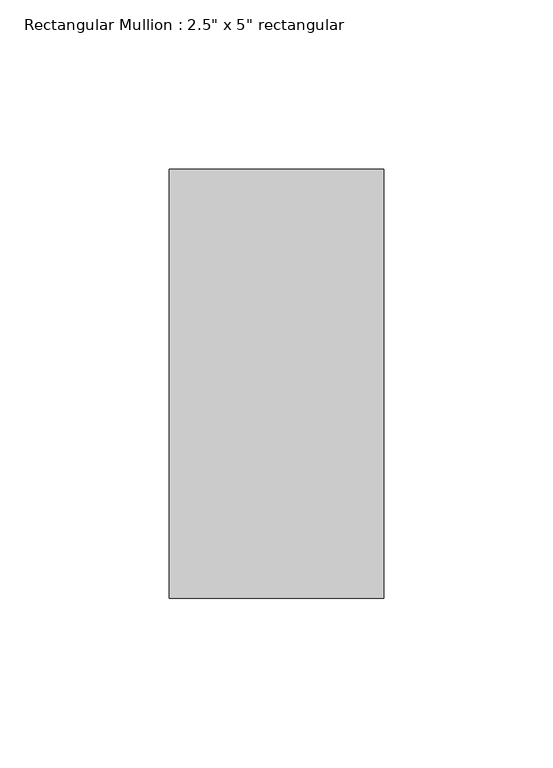
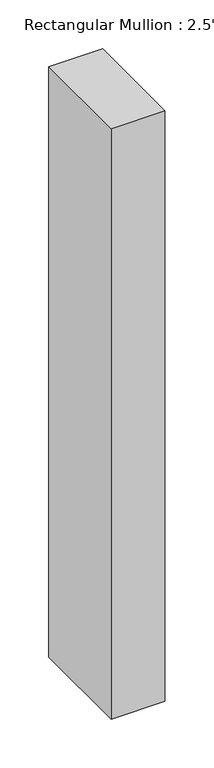
"""IFC4 building model written with IfcOpenShell, lengths in millimetres: member geometry."""

from ifc_helpers import new_model, si_unit, frame, origin, place, context, project, spatial, polyline, outline, extrude, source, transform, mapped, element, save


def member_e61db9c9(model_context):
    return source(origin(), model_context, "Body", "SweptSolid", [
        extrude(outline(polyline([(0.0, 63.5), (0.0, -63.5), (-63.5, -63.5), (-63.5, 63.5), (0.0, 63.5)])), frame((0.0, 0.0, -736.2967564), z_axis=(0.0, 0.0, 1.0), x_axis=(1.0, 0.0, 0.0)), (0.0, 0.0, 1.0), 736.2967564),
    ])


if __name__ == "__main__":
    model = new_model("IFC4")
    model_context = context("Model", 3, world=origin())
    ifc_project = project(units=[si_unit("LENGTHUNIT", "METRE", prefix="MILLI")], contexts=[model_context])
    site = spatial("IfcSite", under=ifc_project)
    building = spatial("IfcBuilding", under=site)
    placement = place(None, origin())
    member_shape = member_e61db9c9(model_context)
    element("IfcMember", 1, ObjectType="Rectangular Mullion : 2.5\" x 5\" rectangular", at=placement, inside=building, context=model_context, shape_type="MappedRepresentation", body=[
        mapped(member_shape, transform((0.0, 0.0, 0.0), x_axis=(1.0, 0.0, 0.0), y_axis=(0.0, 1.0, 0.0), z_axis=(0.0, 0.0, 1.0))),
    ])
    save(model, "model.ifc")

# Revit data of these elements
# Type "Rectangular Mullion : 2.5\" x 5\" rectangular"
#   built-in parameter 1007304 = 0.416667 (stored number, unit not read)
#   built-in parameter 1007301 = 0.104167 (stored number, unit not read)
#   built-in parameter 1007300 = 0.104167 (stored number, unit not read)
# Element 1 (IfcMember, "Rectangular Mullion : 2.5\" x 5\" rectangular")
#   Materials on its faces: "Aluminum"
# Materials
#   "Aluminum": class "Metal", colour RGB 247 247 247, transparency 0, Description = "Aluminum 6061", Cost = 0
